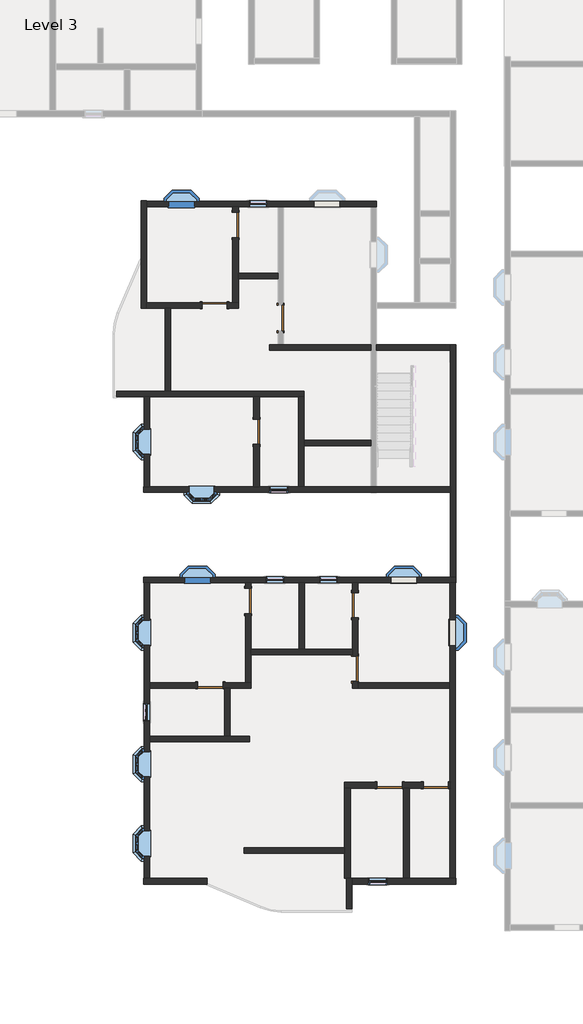
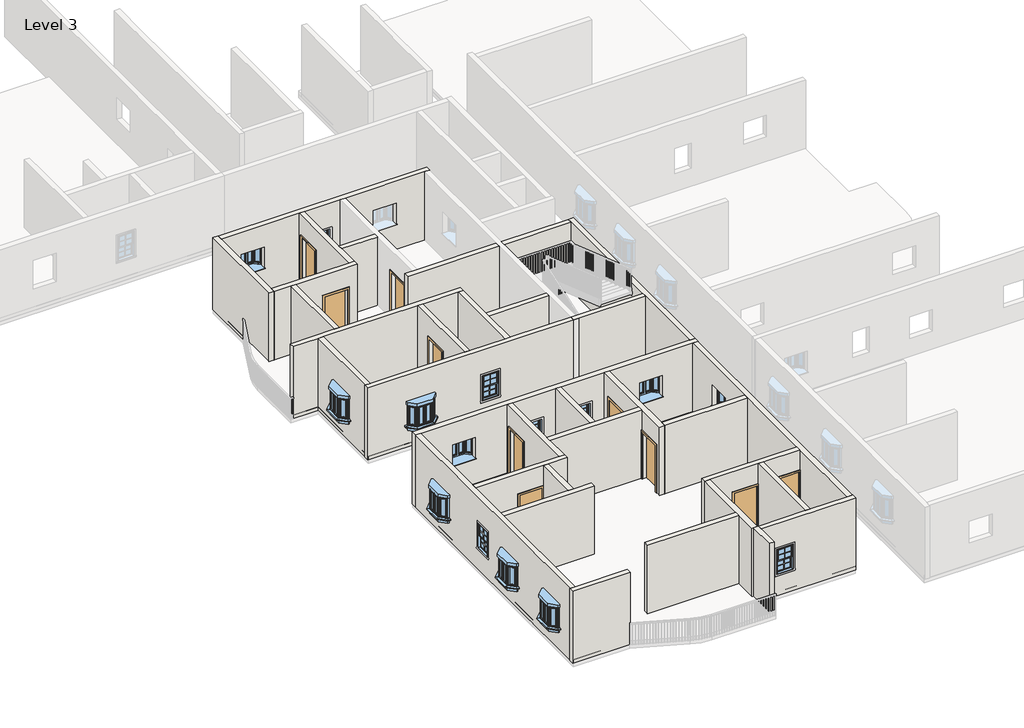
# One storey, part 1 of 14: 32 walls, 15 windows, 10 doors.
# Revit data of these elements (continued)
# Element 54 (IfcWindow, "Window-Double-Hung : 26\" x 42\"") (continued)
#   Window Inset = 0' - 0"
#   Interior Wall Closure = 0' - 1 1/2"
#   Frame Extension = 0' - 1 1/4"
#   Exterior Wall Closure = 0' - 0 1/2"
#   Interior Trim Visibility = yes
#   Indicator Visibility = yes
#   Exterior Trim Visibility = yes
#   Phase Created = New Construction
#   Materials on its faces: "Wood - Stained", "Glass", "Clad - White"
# Element 55 (IfcWindow, "Window-Double-Hung : 26\" x 42\"")
#   Mark = "161"
#   Window Inset = 0' - 0"
#   Interior Wall Closure = 0' - 1 1/2"
#   Frame Extension = 0' - 1 1/4"
#   Exterior Wall Closure = 0' - 0 1/2"
#   Interior Trim Visibility = yes
#   Indicator Visibility = yes
#   Exterior Trim Visibility = yes
#   Phase Created = New Construction
#   Materials on its faces: "Wood - Stained", "Glass", "Clad - White"
# Element 56 (IfcWindow, "Window-Double-Hung : 26\" x 42\"")
#   Mark = "162"
#   Window Inset = 0' - 0"
#   Interior Wall Closure = 0' - 1 1/2"
#   Frame Extension = 0' - 1 1/4"
#   Exterior Wall Closure = 0' - 0 1/2"
#   Interior Trim Visibility = yes
#   Indicator Visibility = yes
#   Exterior Trim Visibility = yes
#   Phase Created = New Construction
#   Materials on its faces: "Wood - Stained", "Glass", "Clad - White"
# Element 57 (IfcWindow, "Window-Double-Hung : 26\" x 42\"")
#   Mark = "163"
#   Window Inset = 0' - 0"
#   Interior Wall Closure = 0' - 1 1/2"
#   Frame Extension = 0' - 1 1/4"
#   Exterior Wall Closure = 0' - 0 1/2"
#   Interior Trim Visibility = yes
#   Indicator Visibility = yes
#   Exterior Trim Visibility = yes
#   Phase Created = New Construction
#   Materials on its faces: "Wood - Stained", "Glass", "Clad - White"
# Materials
#   "Door - Panel": class "Wood", colour RGB 210 159 95, transparency 0, Cost = 0
#   "Door - Frame": colour RGB 118 70 51, transparency 0, Cost = 0
#   "Window Frame": colour RGB 249 249 249, transparency 0
#   "Glass": class "Glass", colour RGB 0 128 192, transparency 0.75, Description = "Soda Lime Glass", Cost = 0
#   "Wood - Stained": class "Wood", colour RGB 224 178 126, transparency 0, Cost = 0
#   "Clad - White": class "Wood", colour RGB 242 242 238, transparency 0, Cost = 0
#   "Default Wall": colour RGB 128 128 128, transparency 0, Cost = 0
#   "Earth": class "Generic", colour RGB 97 75 62, transparency 0, Description = "Soil", Cost = 0
#   "Parking Stripe": class "Paint", colour RGB 250 250 91, transparency 0, Cost = 0
#   "Carpet (1)": class "Carpet", colour RGB 124 80 67, transparency 0, Description = "Interior finish", Cost = 0
#   "Softwood, Lumber": class "Wood", colour RGB 223 192 134, transparency 0, Description = "Pinus Echinata", Cost = 0
